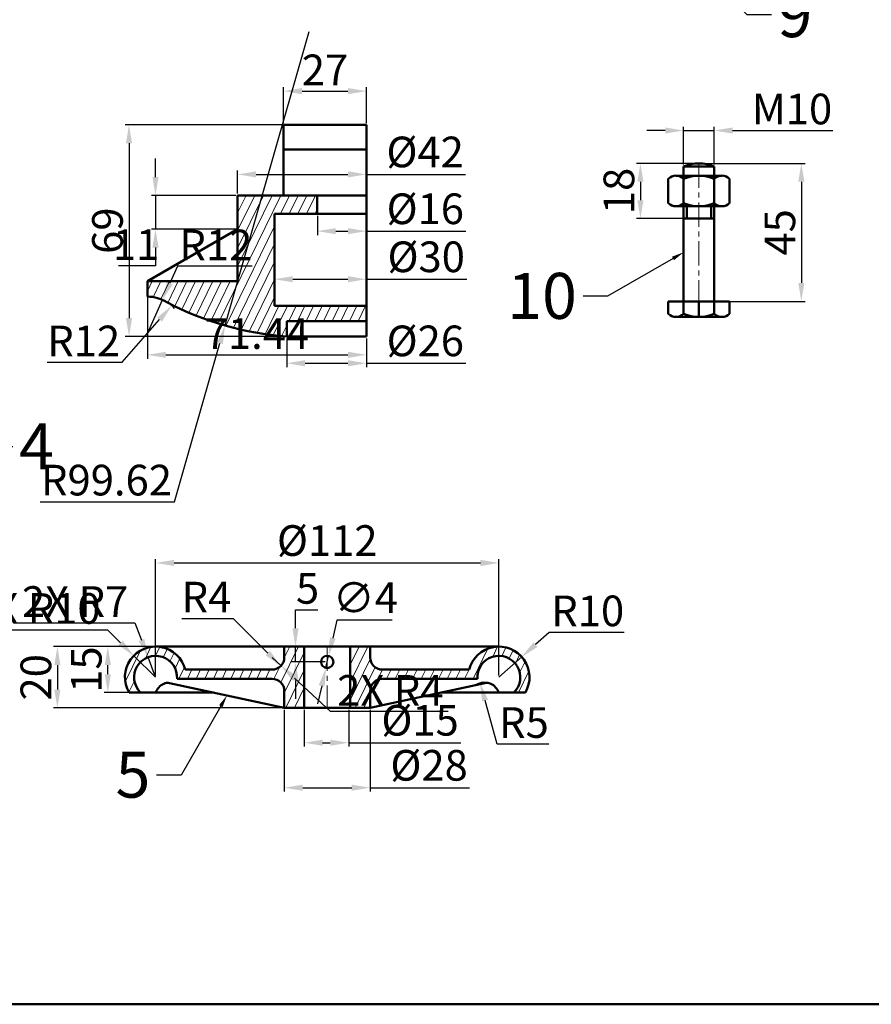
# Model space of a CAD drawing. Units: millimetres. Extents: x 147 to 984, y -369 to 435.
# Tile 3 of 10: x 422 to 699, y -369 to -48. Entities that reach past the tile are written whole.
import ezdxf
from ezdxf import colors
from ezdxf.entities.mleader import LeaderData, LeaderLine
from ezdxf.math import Vec2, Vec3

# ---------------------------------------------------------------- set-up
doc = ezdxf.new("R2010")
doc.units = ezdxf.units.MM
doc.header["$LTSCALE"] = 0.5
doc.linetypes.add('CENTER', pattern=[50.8, 31.75, -6.35, 6.35, -6.35])
for name, color, linetype, lineweight in [('M-CNTR', 1, 'CENTER', 18), ('M-DIMS', 2, 'Continuous', 25), ('M-HATC', 8, 'Continuous', 18), ('M-OUTL', 7, 'Continuous', 50), ('M-TEXT', 7, 'Continuous', 25)]:
    doc.layers.add(name, color=color, linetype=linetype, lineweight=lineweight)
doc.styles.get("Standard").update_dxf_attribs({"font": 'arial.ttf'})
doc.dimstyles.new('ISO-25', dxfattribs={"dimtxt": 10, "dimasz": 6, "dimexe": 1.25, "dimexo": 0.625, "dimtad": 1, "dimtoh": 1, "dimdec": 0, "dimtxsty": 'Standard', "dimcen": 2.5, "dimadec": 0, "dimazin": 0, "dimtfac": 1, "dimtdec": 0, "dimtmove": 0, "dimatfit": 3, "dimfxl": 1, "dimarcsym": 0})

# ---------------------------------------------------------------- blocks, each defined once
blk = doc.blocks.new('*D119')
at = {"layer": 'Defpoints', "color": 0, "ltscale": 0.5, "transparency": 16777216}
for p in [(534.72, -71.63), (507.72, -82.65), (534.72, -82.65)]:
    blk.add_point(p, dxfattribs=at)
at = {"layer": 'M-DIMS', "color": 0, "lineweight": -2, "ltscale": 0.5, "transparency": 16777216}
for p, q in [((507.72, -82.03), (507.72, -70.38)), ((534.72, -82.03), (534.72, -70.38)), ((513.72, -71.63), (528.72, -71.63))]:
    blk.add_line(p, q, dxfattribs=at)
at = {"layer": 'M-DIMS', "color": 0, "ltscale": 0.5, "transparency": 16777216}
for points in [[(513.72, -70.63), (513.72, -72.63), (507.72, -71.63)], [(528.72, -70.63), (528.72, -72.63), (534.72, -71.63)]]:
    blk.add_solid(points, dxfattribs=at)
at = {"layer": 'M-DIMS', "color": 0, "ltscale": 0.5, "transparency": 16777216, "insert": (521.22, -65.99), "char_height": 10, "attachment_point": 5}
blk.add_mtext('27', dxfattribs=at)
blk = doc.blocks.new('*D120')
at = {"layer": 'Defpoints', "color": 0, "ltscale": 0.5, "transparency": 16777216}
for p in [(534.72, -98.78), (492.72, -105.65), (534.72, -105.65)]:
    blk.add_point(p, dxfattribs=at)
at = {"layer": 'M-DIMS', "color": 0, "lineweight": -2, "ltscale": 0.5, "transparency": 16777216}
for p, q in [((492.72, -105.03), (492.72, -97.53)), ((498.72, -98.78), (528.72, -98.78)), ((534.72, -105.03), (534.72, -97.53)), ((534.72, -98.78), (567.07, -98.78))]:
    blk.add_line(p, q, dxfattribs=at)
at = {"layer": 'M-DIMS', "color": 0, "ltscale": 0.5, "transparency": 16777216}
for points in [[(498.72, -97.78), (498.72, -99.78), (492.72, -98.78)], [(528.72, -97.78), (528.72, -99.78), (534.72, -98.78)]]:
    blk.add_solid(points, dxfattribs=at)
at = {"layer": 'M-DIMS', "color": 0, "ltscale": 0.5, "transparency": 16777216, "insert": (553.89, -92.77), "char_height": 10, "attachment_point": 5}
blk.add_mtext('%%C42', dxfattribs=at)
blk = doc.blocks.new('*D121')
at = {"layer": 'Defpoints', "color": 0, "ltscale": 0.5, "transparency": 16777216}
for p in [(518.72, -111.65), (534.72, -111.65), (534.72, -117.31)]:
    blk.add_point(p, dxfattribs=at)
at = {"layer": 'M-DIMS', "color": 0, "lineweight": -2, "ltscale": 0.5, "transparency": 16777216}
for p, q in [((518.72, -112.28), (518.72, -118.56)), ((534.72, -112.28), (534.72, -118.56)), ((524.72, -117.31), (528.72, -117.31)), ((534.72, -117.31), (567.17, -117.31))]:
    blk.add_line(p, q, dxfattribs=at)
at = {"layer": 'M-DIMS', "color": 0, "ltscale": 0.5, "transparency": 16777216}
for points in [[(524.72, -116.31), (524.72, -118.31), (518.72, -117.31)], [(528.72, -116.31), (528.72, -118.31), (534.72, -117.31)]]:
    blk.add_solid(points, dxfattribs=at)
at = {"layer": 'M-DIMS', "color": 0, "ltscale": 0.5, "transparency": 16777216, "insert": (553.94, -111.3), "char_height": 10, "attachment_point": 5}
blk.add_mtext('%%C16', dxfattribs=at)
blk = doc.blocks.new('*D122')
at = {"layer": 'Defpoints', "color": 0, "ltscale": 0.5, "transparency": 16777216}
for p in [(492.72, -105.65), (465.91, -116.65), (492.72, -116.65)]:
    blk.add_point(p, dxfattribs=at)
at = {"layer": 'M-DIMS', "color": 0, "lineweight": -2, "ltscale": 0.5, "transparency": 16777216}
for p, q in [((465.91, -99.65), (465.91, -93.65)), ((492.09, -105.65), (464.66, -105.65)), ((465.91, -105.65), (465.91, -116.65)), ((492.09, -116.65), (464.66, -116.65)), ((465.91, -122.65), (465.91, -128.65)), ((465.91, -128.65), (453.83, -128.65))]:
    blk.add_line(p, q, dxfattribs=at)
at = {"layer": 'M-DIMS', "color": 0, "ltscale": 0.5, "transparency": 16777216}
for points in [[(464.91, -99.65), (466.91, -99.65), (465.91, -105.65)], [(464.91, -122.65), (466.91, -122.65), (465.91, -116.65)]]:
    blk.add_solid(points, dxfattribs=at)
at = {"layer": 'M-DIMS', "color": 0, "ltscale": 0.5, "transparency": 16777216, "insert": (459.56, -123.01), "char_height": 10, "attachment_point": 5}
blk.add_mtext('11', dxfattribs=at)
blk = doc.blocks.new('*D123')
at = {"layer": 'Defpoints', "color": 0, "ltscale": 0.5, "transparency": 16777216}
for p in [(504.72, -133.8), (534.72, -132.98), (534.72, -133.8)]:
    blk.add_point(p, dxfattribs=at)
at = {"layer": 'M-DIMS', "color": 0, "lineweight": -2, "ltscale": 0.5, "transparency": 16777216}
for p, q in [((504.72, -133.18), (504.72, -131.73)), ((510.72, -132.98), (528.72, -132.98)), ((534.72, -133.18), (534.72, -131.73)), ((534.72, -132.98), (567.45, -132.98))]:
    blk.add_line(p, q, dxfattribs=at)
at = {"layer": 'M-DIMS', "color": 0, "ltscale": 0.5, "transparency": 16777216}
for points in [[(510.72, -131.98), (510.72, -133.98), (504.72, -132.98)], [(528.72, -131.98), (528.72, -133.98), (534.72, -132.98)]]:
    blk.add_solid(points, dxfattribs=at)
at = {"layer": 'M-DIMS', "color": 0, "ltscale": 0.5, "transparency": 16777216, "insert": (554.24, -126.97), "char_height": 10, "attachment_point": 5}
blk.add_mtext('%%C30', dxfattribs=at)
blk = doc.blocks.new('*D124')
at = {"layer": 'Defpoints', "color": 0, "ltscale": 0.5, "transparency": 16777216}
for p in [(508.72, -151.65), (534.72, -151.65), (534.72, -160.4)]:
    blk.add_point(p, dxfattribs=at)
at = {"layer": 'M-DIMS', "color": 0, "lineweight": -2, "ltscale": 0.5, "transparency": 16777216}
for p, q in [((508.72, -152.28), (508.72, -161.65)), ((534.72, -152.28), (534.72, -161.65)), ((514.72, -160.4), (528.72, -160.4)), ((534.72, -160.4), (567.17, -160.4))]:
    blk.add_line(p, q, dxfattribs=at)
at = {"layer": 'M-DIMS', "color": 0, "ltscale": 0.5, "transparency": 16777216}
for points in [[(514.72, -159.4), (514.72, -161.4), (508.72, -160.4)], [(528.72, -159.4), (528.72, -161.4), (534.72, -160.4)]]:
    blk.add_solid(points, dxfattribs=at)
at = {"layer": 'M-DIMS', "color": 0, "ltscale": 0.5, "transparency": 16777216, "insert": (553.94, -154.39), "char_height": 10, "attachment_point": 5}
blk.add_mtext('%%C26', dxfattribs=at)
blk = doc.blocks.new('*D125')
at = {"layer": 'Defpoints', "color": 0, "ltscale": 0.5, "transparency": 16777216}
for p in [(471.19, -141.64), (463.27, -150.65)]:
    blk.add_point(p, dxfattribs=at)
at = {"layer": 'M-DIMS', "color": 0, "lineweight": -2, "ltscale": 0.5, "transparency": 16777216}
for p, q in [((455.01, -160.07), (467.23, -146.14)), ((430.6, -160.07), (455.01, -160.07))]:
    blk.add_line(p, q, dxfattribs=at)
blk.add_arc((463.27, -150.65), 12, 42.7638, 55.0883, dxfattribs=at)
at = {"layer": 'M-DIMS', "color": 0, "ltscale": 0.5, "transparency": 16777216}
blk.add_solid([(466.48, -145.49), (467.98, -146.8), (471.19, -141.64)], dxfattribs=at)
at = {"layer": 'M-DIMS', "color": 0, "ltscale": 0.5, "transparency": 16777216, "insert": (442.49, -154.42), "char_height": 10, "attachment_point": 5}
blk.add_mtext('R12', dxfattribs=at)
blk = doc.blocks.new('*D126')
at = {"layer": 'Defpoints', "color": 0, "ltscale": 0.5, "transparency": 16777216}
for p in [(577.95, -225.53), (465.95, -262.83), (577.95, -262.83)]:
    blk.add_point(p, dxfattribs=at)
at = {"layer": 'M-DIMS', "color": 0, "lineweight": -2, "ltscale": 0.5, "transparency": 16777216}
for p, q in [((465.95, -262.2), (465.95, -224.28)), ((577.95, -262.2), (577.95, -224.28)), ((471.95, -225.53), (571.95, -225.53))]:
    blk.add_line(p, q, dxfattribs=at)
at = {"layer": 'M-DIMS', "color": 0, "ltscale": 0.5, "transparency": 16777216}
for points in [[(471.95, -224.53), (471.95, -226.53), (465.95, -225.53)], [(571.95, -224.53), (571.95, -226.53), (577.95, -225.53)]]:
    blk.add_solid(points, dxfattribs=at)
at = {"layer": 'M-DIMS', "color": 0, "ltscale": 0.5, "transparency": 16777216, "insert": (521.95, -219.52), "char_height": 10, "attachment_point": 5}
blk.add_mtext('%%C112', dxfattribs=at)
blk = doc.blocks.new('*D127')
at = {"layer": 'Defpoints', "color": 0, "ltscale": 0.5, "transparency": 16777216}
for p in [(514.45, -272.83), (528.95, -272.83), (528.95, -284.17)]:
    blk.add_point(p, dxfattribs=at)
at = {"layer": 'M-DIMS', "color": 0, "lineweight": -2, "ltscale": 0.5, "transparency": 16777216}
for p, q in [((514.45, -273.45), (514.45, -285.42)), ((528.95, -273.45), (528.95, -285.42)), ((520.45, -284.17), (522.95, -284.17)), ((528.95, -284.17), (565.5, -284.17))]:
    blk.add_line(p, q, dxfattribs=at)
at = {"layer": 'M-DIMS', "color": 0, "ltscale": 0.5, "transparency": 16777216}
for points in [[(520.45, -283.17), (520.45, -285.17), (514.45, -284.17)], [(522.95, -283.17), (522.95, -285.17), (528.95, -284.17)]]:
    blk.add_solid(points, dxfattribs=at)
at = {"layer": 'M-DIMS', "color": 0, "ltscale": 0.5, "transparency": 16777216, "insert": (552.24, -278.15), "char_height": 10, "attachment_point": 5}
blk.add_mtext('%%C15', dxfattribs=at)
blk = doc.blocks.new('*D128')
at = {"layer": 'Defpoints', "color": 0, "ltscale": 0.5, "transparency": 16777216}
for p in [(507.95, -272.83), (535.95, -272.83), (535.95, -298.85)]:
    blk.add_point(p, dxfattribs=at)
at = {"layer": 'M-DIMS', "color": 0, "lineweight": -2, "ltscale": 0.5, "transparency": 16777216}
for p, q in [((507.95, -273.45), (507.95, -300.1)), ((535.95, -273.45), (535.95, -300.1)), ((513.95, -298.85), (529.95, -298.85)), ((535.95, -298.85), (568.42, -298.85))]:
    blk.add_line(p, q, dxfattribs=at)
at = {"layer": 'M-DIMS', "color": 0, "ltscale": 0.5, "transparency": 16777216}
for points in [[(513.95, -297.85), (513.95, -299.85), (507.95, -298.85)], [(529.95, -297.85), (529.95, -299.85), (535.95, -298.85)]]:
    blk.add_solid(points, dxfattribs=at)
at = {"layer": 'M-DIMS', "color": 0, "ltscale": 0.5, "transparency": 16777216, "insert": (555.18, -292.84), "char_height": 10, "attachment_point": 5}
blk.add_mtext('%%C28', dxfattribs=at)
blk = doc.blocks.new('*D129')
at = {"layer": 'Defpoints', "color": 0, "ltscale": 0.5, "transparency": 16777216}
for p in [(521.95, -252.83), (511.59, -257.83), (521.95, -257.83)]:
    blk.add_point(p, dxfattribs=at)
at = {"layer": 'M-DIMS', "color": 0, "lineweight": -2, "ltscale": 0.5, "transparency": 16777216}
for p, q in [((511.59, -246.83), (511.59, -240.83)), ((511.59, -240.83), (518.84, -240.83)), ((521.32, -252.83), (510.34, -252.83)), ((511.59, -257.83), (511.59, -252.83)), ((521.32, -257.83), (510.34, -257.83)), ((511.59, -263.83), (511.59, -269.83))]:
    blk.add_line(p, q, dxfattribs=at)
at = {"layer": 'M-DIMS', "color": 0, "ltscale": 0.5, "transparency": 16777216}
for points in [[(510.59, -246.83), (512.59, -246.83), (511.59, -252.83)], [(510.59, -263.83), (512.59, -263.83), (511.59, -257.83)]]:
    blk.add_solid(points, dxfattribs=at)
at = {"layer": 'M-DIMS', "color": 0, "ltscale": 0.5, "transparency": 16777216, "insert": (515.53, -235.12), "char_height": 10, "attachment_point": 5}
blk.add_mtext('5', dxfattribs=at)
blk = doc.blocks.new('*D130')
at = {"layer": 'Defpoints', "color": 0, "ltscale": 0.5, "transparency": 16777216}
for p in [(522.39, -255.88), (521.5, -259.77)]:
    blk.add_point(p, dxfattribs=at)
at = {"layer": 'M-DIMS', "color": 0, "lineweight": -2, "ltscale": 0.5, "transparency": 16777216}
for p, q in [((525.08, -244.18), (523.74, -250.03)), ((543.1, -244.18), (525.08, -244.18)), ((521.5, -259.77), (522.39, -255.88)), ((520.15, -265.62), (518.81, -271.47))]:
    blk.add_line(p, q, dxfattribs=at)
at = {"layer": 'M-DIMS', "color": 0, "ltscale": 0.5, "transparency": 16777216}
for points in [[(522.77, -249.8), (524.71, -250.25), (522.39, -255.88)], [(519.18, -265.4), (521.13, -265.85), (521.5, -259.77)]]:
    blk.add_solid(points, dxfattribs=at)
at = {"layer": 'M-DIMS', "color": 0, "ltscale": 0.5, "transparency": 16777216, "insert": (534.41, -238.17), "char_height": 10, "attachment_point": 5}
blk.add_mtext('∅4', dxfattribs=at)
blk = doc.blocks.new('*D131')
at = {"layer": 'Defpoints', "color": 0, "ltscale": 0.5, "transparency": 16777216}
for p in [(503.95, -256.33), (506.77, -259.15)]:
    blk.add_point(p, dxfattribs=at)
at = {"layer": 'M-DIMS', "color": 0, "lineweight": -2, "ltscale": 0.5, "transparency": 16777216}
for p, q in [((474.51, -243.6), (491.22, -243.6)), ((491.22, -243.6), (502.53, -254.91))]:
    blk.add_line(p, q, dxfattribs=at)
at = {"layer": 'M-DIMS', "color": 0, "ltscale": 0.5, "transparency": 16777216}
blk.add_solid([(503.24, -254.2), (501.83, -255.62), (506.77, -259.15)], dxfattribs=at)
at = {"layer": 'M-DIMS', "color": 0, "ltscale": 0.5, "transparency": 16777216, "insert": (482.55, -237.97), "char_height": 10, "attachment_point": 5}
blk.add_mtext('R4', dxfattribs=at)
blk = doc.blocks.new('*D132')
at = {"layer": 'Defpoints', "color": 0, "ltscale": 0.5, "transparency": 16777216}
for p in [(571.83, -264.63), (573.17, -269.45)]:
    blk.add_point(p, dxfattribs=at)
at = {"layer": 'M-DIMS', "color": 0, "lineweight": -2, "ltscale": 0.5, "transparency": 16777216}
for p, q in [((577.41, -284.59), (573.44, -270.41)), ((594.23, -284.59), (577.41, -284.59))]:
    blk.add_line(p, q, dxfattribs=at)
blk.add_arc((573.17, -269.45), 5, 72.0675, 119.9371, dxfattribs=at)
at = {"layer": 'M-DIMS', "color": 0, "ltscale": 0.5, "transparency": 16777216}
blk.add_solid([(574.41, -270.14), (572.48, -270.68), (571.83, -264.63)], dxfattribs=at)
at = {"layer": 'M-DIMS', "color": 0, "ltscale": 0.5, "transparency": 16777216, "insert": (586.13, -278.88), "char_height": 10, "attachment_point": 5}
blk.add_mtext('R5', dxfattribs=at)
blk = doc.blocks.new('*D133')
at = {"layer": 'Defpoints', "color": 0, "ltscale": 0.5, "transparency": 16777216}
for p in [(585.41, -256.18), (577.95, -262.83)]:
    blk.add_point(p, dxfattribs=at)
at = {"layer": 'M-DIMS', "color": 0, "lineweight": -2, "ltscale": 0.5, "transparency": 16777216}
for p, q in [((594.38, -248.19), (589.9, -252.18)), ((618.86, -248.19), (594.38, -248.19)), ((577.95, -262.83), (585.41, -256.18))]:
    blk.add_line(p, q, dxfattribs=at)
at = {"layer": 'M-DIMS', "color": 0, "ltscale": 0.5, "transparency": 16777216}
blk.add_solid([(589.23, -251.44), (590.56, -252.93), (585.41, -256.18)], dxfattribs=at)
at = {"layer": 'M-DIMS', "color": 0, "ltscale": 0.5, "transparency": 16777216, "insert": (606.93, -242.46), "char_height": 10, "attachment_point": 5}
blk.add_mtext('R10', dxfattribs=at)
blk = doc.blocks.new('*D134')
at = {"layer": 'Defpoints', "color": 0, "ltscale": 0.5, "transparency": 16777216}
for p in [(507.95, -252.83), (433.9, -272.83), (507.95, -272.83)]:
    blk.add_point(p, dxfattribs=at)
at = {"layer": 'M-DIMS', "color": 0, "lineweight": -2, "ltscale": 0.5, "transparency": 16777216}
for p, q in [((507.32, -252.83), (432.65, -252.83)), ((433.9, -258.83), (433.9, -266.83)), ((507.32, -272.83), (432.65, -272.83))]:
    blk.add_line(p, q, dxfattribs=at)
at = {"layer": 'M-DIMS', "color": 0, "ltscale": 0.5, "transparency": 16777216}
for points in [[(432.9, -258.83), (434.9, -258.83), (433.9, -252.83)], [(432.9, -266.83), (434.9, -266.83), (433.9, -272.83)]]:
    blk.add_solid(points, dxfattribs=at)
at = {"layer": 'M-DIMS', "color": 0, "ltscale": 0.5, "transparency": 16777216, "insert": (428.17, -262.83), "char_height": 10, "attachment_point": 5, "rotation": 90}
blk.add_mtext('20', dxfattribs=at)
blk = doc.blocks.new('*D135')
at = {"layer": 'Defpoints', "color": 0, "ltscale": 0.5, "transparency": 16777216}
for p in [(450.36, -252.83), (465.99, -252.83), (465.99, -267.83)]:
    blk.add_point(p, dxfattribs=at)
at = {"layer": 'M-DIMS', "color": 0, "lineweight": -2, "ltscale": 0.5, "transparency": 16777216}
for p, q in [((465.37, -252.83), (449.11, -252.83)), ((450.36, -261.83), (450.36, -258.83)), ((465.37, -267.83), (449.11, -267.83))]:
    blk.add_line(p, q, dxfattribs=at)
at = {"layer": 'M-DIMS', "color": 0, "ltscale": 0.5, "transparency": 16777216}
for points in [[(449.36, -258.83), (451.36, -258.83), (450.36, -252.83)], [(449.36, -261.83), (451.36, -261.83), (450.36, -267.83)]]:
    blk.add_solid(points, dxfattribs=at)
at = {"layer": 'M-DIMS', "color": 0, "ltscale": 0.5, "transparency": 16777216, "insert": (444.63, -260.33), "char_height": 10, "attachment_point": 5, "rotation": 90}
blk.add_mtext('15', dxfattribs=at)
blk = doc.blocks.new('*D136')
at = {"layer": 'Defpoints', "color": 0, "ltscale": 0.5, "transparency": 16777216}
for p in [(643.24, -95.2), (643.24, -140.2), (676.65, -140.2)]:
    blk.add_point(p, dxfattribs=at)
at = {"layer": 'M-DIMS', "color": 0, "lineweight": -2, "ltscale": 0.5, "transparency": 16777216}
for p, q in [((643.87, -95.2), (677.9, -95.2)), ((676.65, -101.2), (676.65, -134.2)), ((643.87, -140.2), (677.9, -140.2))]:
    blk.add_line(p, q, dxfattribs=at)
at = {"layer": 'M-DIMS', "color": 0, "ltscale": 0.5, "transparency": 16777216}
for points in [[(675.65, -101.2), (677.65, -101.2), (676.65, -95.2)], [(675.65, -134.2), (677.65, -134.2), (676.65, -140.2)]]:
    blk.add_solid(points, dxfattribs=at)
at = {"layer": 'M-DIMS', "color": 0, "ltscale": 0.5, "transparency": 16777216, "insert": (670.94, -117.7), "char_height": 10, "attachment_point": 5, "rotation": 90}
blk.add_mtext('45', dxfattribs=at)
blk = doc.blocks.new('*D137')
at = {"layer": 'Defpoints', "color": 0, "ltscale": 0.5, "transparency": 16777216}
for p in [(643.24, -95.2), (624.14, -113.2), (643.24, -113.2)]:
    blk.add_point(p, dxfattribs=at)
at = {"layer": 'M-DIMS', "color": 0, "lineweight": -2, "ltscale": 0.5, "transparency": 16777216}
for p, q in [((642.62, -95.2), (622.89, -95.2)), ((624.14, -101.2), (624.14, -107.2)), ((642.62, -113.2), (622.89, -113.2))]:
    blk.add_line(p, q, dxfattribs=at)
at = {"layer": 'M-DIMS', "color": 0, "ltscale": 0.5, "transparency": 16777216}
for points in [[(623.14, -101.2), (625.14, -101.2), (624.14, -95.2)], [(623.14, -107.2), (625.14, -107.2), (624.14, -113.2)]]:
    blk.add_solid(points, dxfattribs=at)
at = {"layer": 'M-DIMS', "color": 0, "ltscale": 0.5, "transparency": 16777216, "insert": (618.41, -104.2), "char_height": 10, "attachment_point": 5, "rotation": 90}
blk.add_mtext('18', dxfattribs=at)
blk = doc.blocks.new('*D138')
at = {"layer": 'Defpoints', "color": 0, "ltscale": 0.5, "transparency": 16777216}
for p in [(648.24, -84.48), (638.24, -96.2), (648.24, -96.2)]:
    blk.add_point(p, dxfattribs=at)
at = {"layer": 'M-DIMS', "color": 0, "lineweight": -2, "ltscale": 0.5, "transparency": 16777216}
for p, q in [((638.24, -95.58), (638.24, -83.23)), ((648.24, -95.58), (648.24, -83.23)), ((632.24, -84.48), (626.24, -84.48)), ((638.24, -84.48), (648.24, -84.48)), ((654.24, -84.48), (686.96, -84.48))]:
    blk.add_line(p, q, dxfattribs=at)
at = {"layer": 'M-DIMS', "color": 0, "ltscale": 0.5, "transparency": 16777216}
for points in [[(632.24, -83.48), (632.24, -85.48), (638.24, -84.48)], [(654.24, -83.48), (654.24, -85.48), (648.24, -84.48)]]:
    blk.add_solid(points, dxfattribs=at)
at = {"layer": 'M-DIMS', "color": 0, "ltscale": 0.5, "transparency": 16777216, "insert": (673.6, -78.75), "char_height": 10, "attachment_point": 5}
blk.add_mtext('M10', dxfattribs=at)
blk = doc.blocks.new('*D144')
at = {"layer": 'Defpoints', "color": 0, "ltscale": 0.5, "transparency": 16777216}
for p in [(507.72, -82.65), (457.27, -151.65), (508.72, -151.65)]:
    blk.add_point(p, dxfattribs=at)
at = {"layer": 'M-DIMS', "color": 0, "lineweight": -2, "ltscale": 0.5, "transparency": 16777216}
for p, q in [((507.09, -82.65), (456.02, -82.65)), ((457.27, -88.65), (457.27, -145.65)), ((508.09, -151.65), (456.02, -151.65))]:
    blk.add_line(p, q, dxfattribs=at)
at = {"layer": 'M-DIMS', "color": 0, "ltscale": 0.5, "transparency": 16777216}
for points in [[(456.27, -88.65), (458.27, -88.65), (457.27, -82.65)], [(456.27, -145.65), (458.27, -145.65), (457.27, -151.65)]]:
    blk.add_solid(points, dxfattribs=at)
at = {"layer": 'M-DIMS', "color": 0, "ltscale": 0.5, "transparency": 16777216, "insert": (451.54, -117.15), "char_height": 10, "attachment_point": 5, "rotation": 90}
blk.add_mtext('69', dxfattribs=at)
blk = doc.blocks.new('*D145')
at = {"layer": 'Defpoints', "color": 0, "ltscale": 0.5, "transparency": 16777216}
for p in [(463.27, -133.65), (534.72, -151.65), (534.72, -157.65)]:
    blk.add_point(p, dxfattribs=at)
at = {"layer": 'M-DIMS', "color": 0, "lineweight": -2, "ltscale": 0.5, "transparency": 16777216}
for p, q in [((463.27, -134.28), (463.27, -158.9)), ((534.72, -152.28), (534.72, -158.9)), ((469.27, -157.65), (528.72, -157.65))]:
    blk.add_line(p, q, dxfattribs=at)
at = {"layer": 'M-DIMS', "color": 0, "ltscale": 0.5, "transparency": 16777216}
for points in [[(469.27, -156.65), (469.27, -158.65), (463.27, -157.65)], [(528.72, -156.65), (528.72, -158.65), (534.72, -157.65)]]:
    blk.add_solid(points, dxfattribs=at)
at = {"layer": 'M-DIMS', "color": 0, "ltscale": 0.5, "transparency": 16777216, "insert": (499, -152.01), "char_height": 10, "attachment_point": 5}
blk.add_mtext('71.44', dxfattribs=at)
blk = doc.blocks.new('*D187')
at = {"layer": 'Defpoints', "color": 0, "ltscale": 0.5, "transparency": 16777216}
for p in [(458.81, -255.82), (465.95, -262.83)]:
    blk.add_point(p, dxfattribs=at)
at = {"layer": 'M-DIMS', "color": 0, "lineweight": -2, "ltscale": 0.5, "transparency": 16777216}
for p, q in [((404.11, -247.4), (450.26, -247.4)), ((450.26, -247.4), (454.54, -251.61)), ((465.95, -262.83), (458.81, -255.82))]:
    blk.add_line(p, q, dxfattribs=at)
at = {"layer": 'M-DIMS', "color": 0, "ltscale": 0.5, "transparency": 16777216}
blk.add_solid([(455.24, -250.9), (453.83, -252.32), (458.81, -255.82)], dxfattribs=at)
at = {"layer": 'M-DIMS', "color": 0, "ltscale": 0.5, "transparency": 16777216, "insert": (426.87, -241.67), "char_height": 10, "attachment_point": 5}
blk.add_mtext('2X R10', dxfattribs=at)
blk = doc.blocks.new('*D188')
at = {"layer": 'Defpoints', "color": 0, "ltscale": 0.5, "transparency": 16777216}
for p in [(463.47, -256.28), (465.95, -262.83)]:
    blk.add_point(p, dxfattribs=at)
at = {"layer": 'M-DIMS', "color": 0, "lineweight": -2, "ltscale": 0.5, "transparency": 16777216}
for p, q in [((420.81, -245.06), (459.22, -245.06)), ((459.22, -245.06), (461.34, -250.67)), ((465.95, -262.83), (463.47, -256.28))]:
    blk.add_line(p, q, dxfattribs=at)
at = {"layer": 'M-DIMS', "color": 0, "ltscale": 0.5, "transparency": 16777216}
blk.add_solid([(462.28, -250.31), (460.41, -251.02), (463.47, -256.28)], dxfattribs=at)
at = {"layer": 'M-DIMS', "color": 0, "ltscale": 0.5, "transparency": 16777216, "insert": (439.7, -239.41), "char_height": 10, "attachment_point": 5}
blk.add_mtext('2X R7', dxfattribs=at)
blk = doc.blocks.new('*D189')
at = {"layer": 'Defpoints', "color": 0, "ltscale": 0.5, "transparency": 16777216}
for p in [(503.95, -256.33), (506.88, -259.04)]:
    blk.add_point(p, dxfattribs=at)
at = {"layer": 'M-DIMS', "color": 0, "lineweight": -2, "ltscale": 0.5, "transparency": 16777216}
for p, q in [((503.95, -256.33), (506.88, -259.04)), ((523.05, -274.03), (511.28, -263.12)), ((561.42, -274.03), (523.05, -274.03))]:
    blk.add_line(p, q, dxfattribs=at)
at = {"layer": 'M-DIMS', "color": 0, "ltscale": 0.5, "transparency": 16777216}
blk.add_solid([(511.96, -262.39), (510.6, -263.86), (506.88, -259.04)], dxfattribs=at)
at = {"layer": 'M-DIMS', "color": 0, "ltscale": 0.5, "transparency": 16777216, "insert": (542.54, -268.39), "char_height": 10, "attachment_point": 5}
blk.add_mtext('2X R4', dxfattribs=at)
blk = doc.blocks.new('*D190')
at = {"layer": 'Defpoints', "color": 0, "ltscale": 0.5, "transparency": 16777216}
for p in [(515.99, -52.3), (488.59, -148.08)]:
    blk.add_point(p, dxfattribs=at)
at = {"layer": 'M-DIMS', "color": 0, "lineweight": -2, "ltscale": 0.5, "transparency": 16777216}
for p, q in [((515.99, -52.3), (488.59, -148.08)), ((472.15, -205.55), (486.94, -153.85)), ((428.31, -205.55), (472.15, -205.55))]:
    blk.add_line(p, q, dxfattribs=at)
at = {"layer": 'M-DIMS', "color": 0, "ltscale": 0.5, "transparency": 16777216}
blk.add_solid([(485.98, -153.57), (487.9, -154.12), (488.59, -148.08)], dxfattribs=at)
at = {"layer": 'M-DIMS', "color": 0, "ltscale": 0.5, "transparency": 16777216, "insert": (449.92, -199.81), "char_height": 10, "attachment_point": 5}
blk.add_mtext('R99.62', dxfattribs=at)
blk = doc.blocks.new('*D191')
at = {"layer": 'Defpoints', "color": 0, "ltscale": 0.5, "transparency": 16777216}
for p in [(468.18, -139.7), (463.27, -150.65)]:
    blk.add_point(p, dxfattribs=at)
at = {"layer": 'M-DIMS', "color": 0, "lineweight": -2, "ltscale": 0.5, "transparency": 16777216}
for p, q in [((473.08, -128.75), (470.63, -134.23)), ((497.5, -128.75), (473.08, -128.75)), ((463.27, -150.65), (468.18, -139.7))]:
    blk.add_line(p, q, dxfattribs=at)
at = {"layer": 'M-DIMS', "color": 0, "ltscale": 0.5, "transparency": 16777216}
blk.add_solid([(469.72, -133.82), (471.54, -134.64), (468.18, -139.7)], dxfattribs=at)
at = {"layer": 'M-DIMS', "color": 0, "ltscale": 0.5, "transparency": 16777216, "insert": (485.6, -123.11), "char_height": 10, "attachment_point": 5}
blk.add_mtext('R12', dxfattribs=at)

msp = doc.modelspace()

# ---------------------------------------------------------------- hatches: boundary and pattern name
at = {"layer": 'M-HATC', "ltscale": 0.5}
h = msp.add_hatch(dxfattribs=at)
h.set_pattern_fill('ANSI31', color=256, scale=0.8, angle=199)
h.set_pattern_definition([(244, (-217.7436, 170.283), (2.282937, -1.113463), [])])
h.paths.add_polyline_path([(463.2726, -133.6547), (463.2726, -138.6547, -0.14021832), (469.6187, -140.4701, 0.10314178), (508.7174, -151.6547), (508.7174, -146.6547), (534.7174, -146.6547), (534.7174, -141.6547), (504.7174, -141.6547), (504.7174, -111.6547), (518.7174, -111.6547), (518.7174, -105.6547), (507.7174, -105.6547), (492.7174, -105.6547), (492.7174, -133.6547)])
h = msp.add_hatch(dxfattribs=at)
h.set_pattern_fill('ANSI31', color=256, scale=0.8, angle=199)
h.set_pattern_definition([(244, (-273.2544, -32.9847), (2.282937, -1.113463), [])])
h.paths.add_polyline_path([(503.9465, -260.3255), (475.629, -260.3255, 1.14553919), (457.2863, -267.8255), (461.0475, -267.8255, -1.56487068), (472.9286, -263.3255), (503.9465, -263.3255, -0.41421356), (507.9465, -267.3255), (507.9465, -272.8255), (514.4465, -272.8255), (514.4465, -252.8255), (507.9465, -252.8255), (507.9465, -256.3255, -0.41421356)])
h.paths.add_polyline_path([(529.4465, -272.8255), (535.9465, -272.8255), (535.9465, -267.3255, -0.41421356), (539.9465, -263.3255), (570.9644, -263.3255, -1.56487068), (582.8455, -267.8255), (586.6068, -267.8255, 1.14553919), (568.2641, -260.3255), (539.9465, -260.3255, -0.41421356), (535.9465, -256.3255), (535.9465, -252.8255), (529.4465, -252.8255)])

# ---------------------------------------------------------------- linework, layer by layer
at = {"layer": 'M-CNTR', "ltscale": 0.5}
for p, q in [((643.2406, -95.2039), (643.2406, -140.2039)), ((521.9465, -252.8255), (521.9465, -272.8255))]:
    msp.add_line(p, q, dxfattribs=at)
at = {"layer": 'M-OUTL', "ltscale": 0.5}
for p, q in [((534.7174, -82.6547), (507.7174, -82.6547)), ((507.7174, -82.6547), (507.7174, -90.6547)), ((534.7174, -151.6547), (534.7174, -82.6547)), ((507.7174, -90.6547), (534.7174, -90.6547)), ((507.7174, -90.6547), (507.7174, -105.6547)), ((638.2406, -100.2039), (638.2406, -96.2039)), ((638.2406, -96.2039), (648.2406, -96.2039)), ((648.2406, -96.2039), (648.2406, -100.2039)), ((635.6604, -99.2039), (650.8228, -99.2039)), ((633.2406, -108.2039), (633.2406, -100.2039)), ((638.2406, -100.2039), (638.2406, -108.2039)), ((648.2406, -100.2039), (648.2406, -108.2039)), ((653.2406, -100.2039), (653.2406, -108.2039)), ((507.7174, -105.6547), (492.7174, -105.6547)), ((492.7174, -105.6547), (492.7174, -133.6547)), ((507.7174, -105.6547), (534.7174, -105.6547)), ((518.7174, -105.6547), (518.7174, -111.6547)), ((638.2406, -108.2039), (638.2406, -140.2039)), ((648.2406, -108.2039), (648.2406, -140.2039)), ((534.7174, -111.6547), (504.7174, -111.6547)), ((504.7174, -111.6547), (504.7174, -141.6547)), ((650.8228, -109.2039), (635.6604, -109.2039)), ((639.2406, -109.2039), (639.2406, -113.2039)), ((647.2406, -109.2039), (647.2406, -113.2039)), ((638.2406, -113.2039), (648.2406, -113.2039)), ((492.7174, -116.6547), (463.2726, -133.6547)), ((463.2726, -133.6547), (492.7174, -133.6547)), ((463.2726, -133.6547), (463.2726, -138.6547)), ((633.2406, -144.269), (633.2406, -140.2039)), ((633.2406, -140.2039), (653.2406, -140.2039)), ((638.2406, -140.2039), (638.2406, -144.269)), ((643.2406, -140.2039), (643.2406, -145.269)), ((648.2406, -140.2039), (648.2406, -144.269)), ((653.2406, -140.2039), (653.2406, -144.269)), ((504.7174, -141.6547), (534.7174, -141.6547)), ((508.7174, -151.6547), (508.7174, -146.6547)), ((508.7174, -146.6547), (534.7174, -146.6547)), ((650.8228, -145.269), (635.6604, -145.269)), ((508.7174, -151.6547), (534.7174, -151.6547)), ((521.9465, -252.8255), (465.9465, -252.8255)), ((507.9465, -252.8255), (507.9465, -256.3255)), ((514.4465, -252.8255), (514.4465, -272.8255)), ((521.9465, -252.8255), (577.9465, -252.8255)), ((529.4465, -252.8255), (529.4465, -272.8255)), ((535.9465, -252.8255), (535.9465, -256.3255)), ((503.9465, -263.3255), (472.9286, -263.3255)), ((503.9465, -260.3255), (475.629, -260.3255)), ((539.9465, -260.3255), (568.2641, -260.3255)), ((539.9465, -263.3255), (570.9644, -263.3255)), ((470.5067, -264.7065), (507.9465, -272.8255)), ((573.3863, -264.7065), (535.9465, -272.8255)), ((457.2863, -267.8255), (484.8895, -267.8255)), ((507.9465, -267.3255), (507.9465, -272.8255)), ((535.9465, -267.3255), (535.9465, -272.8255)), ((586.6068, -267.8255), (559.0035, -267.8255)), ((507.9465, -272.8255), (521.9465, -272.8255)), ((535.9465, -272.8255), (521.9465, -272.8255))]:
    msp.add_line(p, q, dxfattribs=at)
msp.add_lwpolyline([(147.3511, 435.3078), (984.0884, 435.3078), (984.0884, -369.4968), (147.3511, -369.4968)], close=True, dxfattribs=at)
msp.add_circle((521.9465, -257.8255), 2, dxfattribs=at)
for centre, radius, start, end in [((643.2406, -108.2039), 13, 67.380135, 112.619865), ((635.7406, -102.8257), 3.6227, 46.362059, 133.637941), ((643.2406, -112.2039), 13, 67.380135, 112.619865), ((650.7406, -102.8255), 3.6226, 46.360394, 133.639606), ((635.7406, -105.5821), 3.6227, 226.362059, 313.637941), ((643.2406, -96.2039), 13, 247.380135, 292.619865), ((650.7406, -105.5823), 3.6226, 226.360394, 313.639606), ((463.2726, -150.6547), 12, 58.072487, 90), ((515.9895, -52.3012), 99.6192, 242.258712, 265.813775), ((635.7406, -141.6473), 3.6227, 226.362059, 313.637941), ((643.2406, -132.269), 13, 247.380135, 292.619865), ((650.7406, -141.6474), 3.6226, 226.360394, 313.639606), ((465.9465, -262.8255), 10, 14.477512, 210), ((577.9465, -262.8255), 10, 330, 165.522488), ((465.9465, -262.8255), 7, 355.903956, 225.584691), ((503.9465, -256.3255), 4, 270, 0), ((539.9465, -256.3255), 4, 180, 270), ((577.9465, -262.8255), 7, 314.415309, 184.096044), ((503.9465, -267.3255), 4, 0, 90), ((539.9465, -267.3255), 4, 90, 180), ((470.7192, -269.4496), 5, 115.094449, 161.045036), ((469.871, -267.6384), 3, 77.764645, 115.094449), ((574.0221, -267.6384), 3, 64.905551, 102.235355), ((573.1738, -269.4496), 5, 18.954964, 64.905551)]:
    msp.add_arc(centre, radius, start, end, dxfattribs=at)

# ---------------------------------------------------------------- dimensions: what is measured, and where the dimension line sits
at = {"layer": 'M-DIMS', "ltscale": 0.5}
for center, mpoint, override, picture, middle in [((515.9895, -52.3012), (488.5911, -148.0787), {"dimdec": 2, "dimlfac": 1, "dimrnd": 0, "dimzin": 0, "dimdsep": 46, "dimlunit": 2}, '*D190', (449.9206, -205.5452)), ((463.2726, -150.6547), (471.1875, -141.6351), {"dimclrd": 0, "dimclre": 0, "dimclrt": 0}, '*D125', (442.4925, -160.0662)), ((503.9465, -256.3255), (506.7749, -259.1539), {"dimclrd": 0, "dimclre": 0, "dimclrt": 0}, '*D131', (482.5513, -243.5975)), ((573.1738, -269.4496), (571.8281, -264.6341), {"dimclrd": 0, "dimclre": 0, "dimclrt": 0}, '*D132', (586.1314, -284.5946))]:
    dim = msp.add_radius_dim(center=center, mpoint=mpoint, dimstyle='ISO-25', override=override, dxfattribs=at)
    dim.commit()
    dim.dimension.update_dxf_attribs({"geometry": picture, "text_midpoint": middle, "dimtype": 164})
for base, p1, p2, override, picture, middle in [((534.7174, -71.6321), (507.7174, -82.6547), (534.7174, -82.6547), {"dimclrd": 0, "dimclre": 0, "dimclrt": 0}, '*D119', (521.2174, -65.9867)), ((534.7174, -157.6547), (463.2726, -133.6547), (534.7174, -151.6547), {"dimdec": 2, "dimlfac": 1, "dimrnd": 0, "dimzin": 0, "dimdsep": 46, "dimlunit": 2}, '*D145', (498.995, -152.0092))]:
    dim = msp.add_linear_dim(base=base, p1=p1, p2=p2, dimstyle='ISO-25', override=override, dxfattribs=at)
    dim.commit()
    dim.dimension.update_dxf_attribs({"geometry": picture, "text_midpoint": middle})
for base, p1, p2, text, picture, middle in [((648.2406, -84.4763), (638.2406, -96.2039), (648.2406, -96.2039), 'M<>', '*D138', (673.601, -78.7456)), ((534.7174, -160.3996), (508.7174, -151.6547), (534.7174, -151.6547), '%%C<>', '*D124', (553.9414, -154.3892)), ((577.9465, -225.5335), (465.9465, -262.8255), (577.9465, -262.8255), '%%C<>', '*D126', (521.9465, -219.5231))]:
    dim = msp.add_linear_dim(base=base, p1=p1, p2=p2, text=text, dimstyle='ISO-25', override={"dimclrd": 0, "dimclre": 0, "dimclrt": 0}, dxfattribs=at)
    dim.commit()
    dim.dimension.update_dxf_attribs({"geometry": picture, "text_midpoint": middle})
for base, p1, p2, override, picture, middle in [((457.2726, -151.6547), (507.7174, -82.6547), (508.7174, -151.6547), {"dimdec": 0, "dimlfac": 1, "dimrnd": 0, "dimzin": 0, "dimdsep": 46, "dimlunit": 2}, '*D144', (451.5419, -117.1547)), ((465.9081, -116.6547), (492.7174, -105.6547), (492.7174, -116.6547), {"dimclrd": 0, "dimclre": 0, "dimclrt": 0}, '*D122', (459.5566, -123.0092)), ((624.1366, -113.2039), (643.2406, -95.2039), (643.2406, -113.2039), {"dimclrd": 0, "dimclre": 0, "dimclrt": 0}, '*D137', (618.4059, -104.2039)), ((676.6485, -140.2039), (643.2406, -95.2039), (643.2406, -140.2039), {"dimclrd": 0, "dimclre": 0, "dimclrt": 0}, '*D136', (670.9382, -117.7039))]:
    dim = msp.add_linear_dim(base=base, p1=p1, p2=p2, angle=90, dimstyle='ISO-25', override=override, dxfattribs=at)
    dim.commit()
    dim.dimension.update_dxf_attribs({"geometry": picture, "text_midpoint": middle})
for base, p1, p2, picture, middle in [((534.7174, -98.7798), (492.7174, -105.6547), (534.7174, -105.6547), '*D120', (553.8936, -98.7798)), ((534.7174, -117.3072), (518.7174, -111.6547), (534.7174, -111.6547), '*D121', (553.9414, -117.3072)), ((534.7174, -132.9794), (504.7174, -133.8013), (534.7174, -133.8013), '*D123', (554.2432, -132.9794)), ((535.9465, -298.8504), (507.9465, -272.8255), (535.9465, -272.8255), '*D128', (555.1841, -298.8504)), ((528.9465103238, -284.1650652448), (514.4465103238, -272.8254663136), (528.9465103238, -272.8254663136), '*D127', (552.2353085407, -284.1650652448))]:
    dim = msp.add_linear_dim(base=base, p1=p1, p2=p2, text='%%C<>', dimstyle='ISO-25', override={"dimclrd": 0, "dimclre": 0, "dimclrt": 0}, dxfattribs=at)
    dim.commit()
    dim.dimension.update_dxf_attribs({"geometry": picture, "text_midpoint": middle, "dimtype": 160})
for center, mpoint, override, picture, middle in [((463.2726, -150.6547), (468.1778, -139.703), {"dimdec": 0, "dimlfac": 1, "dimrnd": 0, "dimzin": 0, "dimdsep": 46, "dimlunit": 2}, '*D191', (485.6043, -123.1059)), ((577.9465, -262.8255), (585.4146, -256.1751), {"dimclrd": 0, "dimclre": 0, "dimclrt": 0}, '*D133', (606.9318, -242.4639))]:
    dim = msp.add_radius_dim(center=center, mpoint=mpoint, dimstyle='ISO-25', override=override, dxfattribs=at)
    dim.commit()
    dim.dimension.update_dxf_attribs({"geometry": picture, "text_midpoint": middle})
for center, mpoint, picture, middle in [((465.9465, -262.8255), (463.4671, -256.2793), '*D188', (439.7002, -239.4084)), ((465.9465, -262.8255), (458.8145, -255.8159), '*D187', (426.8718, -241.6737)), ((503.9465, -256.3255), (506.8799, -259.0449), '*D189', (542.5446, -268.3853))]:
    dim = msp.add_radius_dim(center=center, mpoint=mpoint, text='2X <>', dimstyle='ISO-25', override={"dimdec": 0, "dimlfac": 1, "dimrnd": 0, "dimzin": 0, "dimdsep": 46, "dimlunit": 2}, dxfattribs=at)
    dim.commit()
    dim.dimension.update_dxf_attribs({"geometry": picture, "text_midpoint": middle})
for base, p1, p2, picture, middle in [((511.5863, -257.8255), (521.9465, -252.8255), (521.9465, -257.8255), '*D129', (515.5265, -240.8255)), ((433.9048, -272.8255), (507.9465, -252.8255), (507.9465, -272.8255), '*D134', (433.9048, -262.8255)), ((450.364, -252.8255), (465.9903, -267.8255), (465.9903, -252.8255), '*D135', (450.364, -260.3255))]:
    dim = msp.add_linear_dim(base=base, p1=p1, p2=p2, angle=90, dimstyle='ISO-25', override={"dimclrd": 0, "dimclre": 0, "dimclrt": 0}, dxfattribs=at)
    dim.commit()
    dim.dimension.update_dxf_attribs({"geometry": picture, "text_midpoint": middle, "dimtype": 160})
dim = msp.add_diameter_dim_2p(p1=(521.4982, -259.7746), p2=(522.3948, -255.8763), dimstyle='ISO-25', override={"dimclrd": 0, "dimclre": 0, "dimclrt": 0}, dxfattribs=at)
dim.commit()
dim.dimension.update_dxf_attribs({"geometry": '*D130', "text_midpoint": (534.4065, -238.1712)})

# ---------------------------------------------------------------- leaders
at = {"layer": 'M-TEXT', "ltscale": 0.5}
ml = msp.add_multileader_mtext('Standard', dxfattribs=at)
ml.set_content('9', color=256)
ml.set_leader_properties()
ml.build(insert=Vec2(0, 0))
ctx = ml.context
ctx.base_point, ctx.char_height, ctx.plane_origin = Vec3(666.8716, -46.6451), 15, Vec3(641.1369, -29.0372)
notes = []
notes.append((ctx, [(0, (1, 1, 0), (658.8716, -46.6451), (1, 0), 8, [(0, [(641.1369, -29.0372)], 0, [])])]))
ctx.mtext.insert, ctx.mtext.flow_direction = Vec3(668.8716, -39.0172), 5
ml = msp.add_multileader_mtext('Standard', dxfattribs=at)
ml.set_content('10', color=256)
ml.set_leader_properties()
ml.build(insert=Vec2(0, 0))
ctx = ml.context
ctx.base_point, ctx.char_height, ctx.plane_origin = Vec3(581.3862, -138.5398), 15, Vec3(638.2406, -124.2039)
ctx.text_align_type = 2
notes.append((ctx, [(0, (1, 1, 0), (613.4101, -138.5398), (-1, 0), 8, [(0, [(638.2406, -124.2039)], 0, [])])]))
ctx.mtext.insert, ctx.mtext.alignment, ctx.mtext.flow_direction = Vec3(603.4101, -130.9119), 3, 5
ml = msp.add_multileader_mtext('Standard', dxfattribs=at)
ml.set_content('4', color=256)
ml.set_leader_properties()
ml.build(insert=Vec2(0, 0))
ctx = ml.context
ctx.base_point, ctx.char_height, ctx.plane_origin = Vec3(419.374, -187.5359), 15, Vec3(365.8323, -141.6547)
notes.append((ctx, [(0, (1, 1, 0), (411.374, -187.5359), (1, 0), 8, [(0, [(365.8323, -141.6547)], 0, [])])]))
ctx.mtext.insert, ctx.mtext.flow_direction = Vec3(421.374, -180.0359), 5
ml = msp.add_multileader_mtext('Standard', dxfattribs=at)
ml.set_content('5', color=256)
ml.set_leader_properties()
ml.build(insert=Vec2(0, 0))
ctx = ml.context
ctx.base_point, ctx.char_height, ctx.plane_origin = Vec3(452.2946, -294.7236), 15, Vec3(489.2266, -268.766)
ctx.text_align_type = 2
notes.append((ctx, [(0, (1, 1, 0), (474.24, -294.7236), (-1, 0), 8, [(0, [(489.2266, -268.766)], 0, [])])]))
ctx.mtext.insert, ctx.mtext.alignment, ctx.mtext.flow_direction = Vec3(464.24, -287.0957), 3, 5
for ctx, leaders in notes:
    for number, flags, end, landing, length, lines in leaders:
        leader = LeaderData()
        leader.index, (leader.has_last_leader_line, leader.has_dogleg_vector, leader.attachment_direction) = number, flags
        leader.last_leader_point, leader.dogleg_vector, leader.dogleg_length = Vec3(end), Vec3(landing), length
        for number, points, colour, breaks in lines:
            line = LeaderLine()
            line.index, line.vertices, line.color, line.breaks = number, Vec3.list(points), colors.encode_raw_color(colour), breaks
            leader.lines.append(line)
        ctx.leaders.append(leader)

doc.saveas('drawing.dxf')
